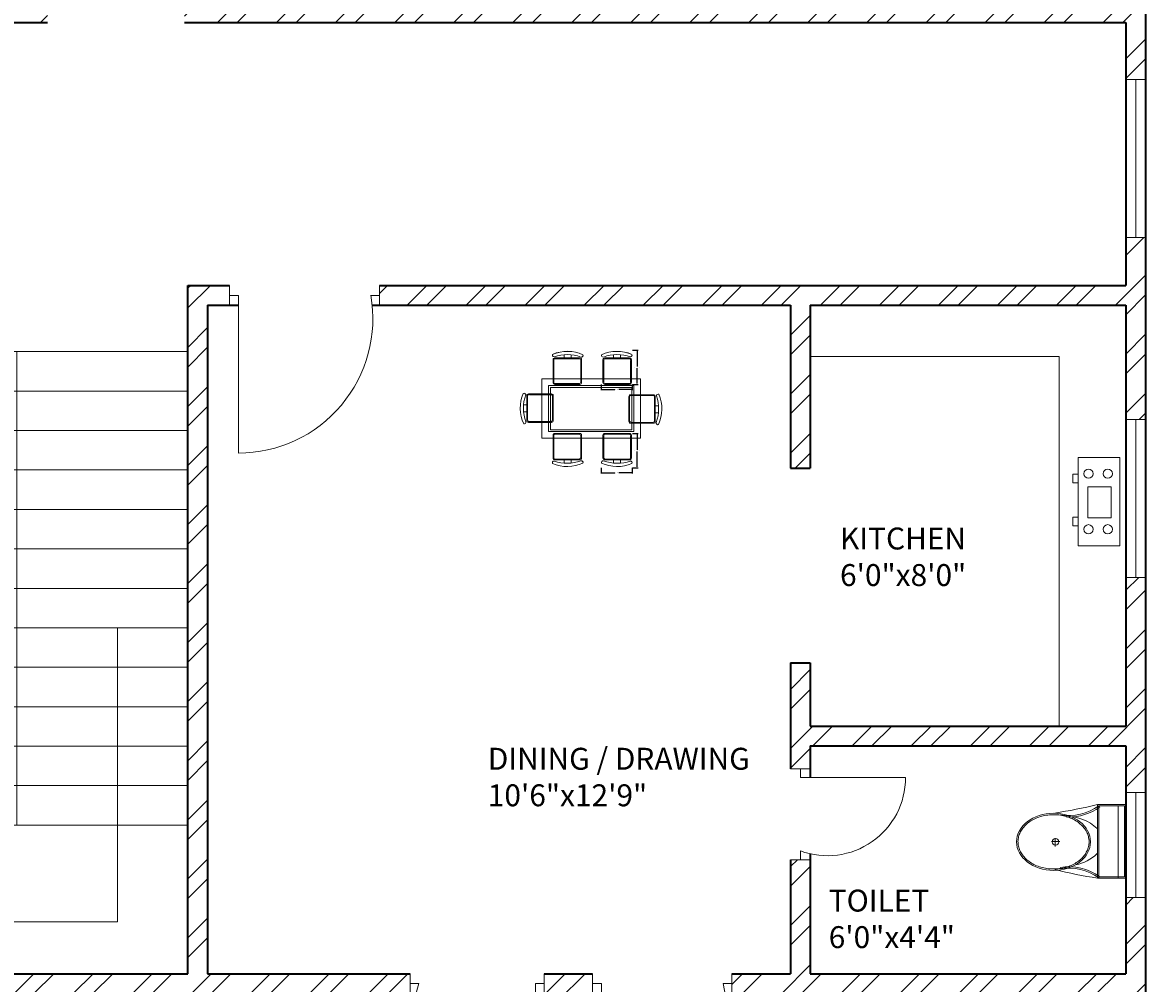
# Model space of a CAD drawing. Units: inches. Extents: x 1944 to 3454, y 1352 to 3055.
# Tile 4 of 17: x 2314 to 2570, y 1681 to 1900. Entities that reach past the tile are written whole.
import ezdxf

# ---------------------------------------------------------------- set-up
doc = ezdxf.new("R2010")
doc.units = ezdxf.units.IN
for name, color, linetype, lineweight in [('A-ANNO-DIMS', 2, 'Continuous', 18), ('A-AREA-IDEN', 7, 'Continuous', 18), ('A-DOOR', 3, 'Continuous', 20), ('A-EQPM', 9, 'Continuous', 18), ('A-FLOR-CASE', 8, 'Continuous', 20), ('A-FLOR-FIXT', 9, 'Continuous', 18), ('A-FLOR-STRS', 7, 'Continuous', 20), ('A-FURN', 8, 'Continuous', 13), ('A-GLAZ', 4, 'Continuous', 18), ('A-WALL', 7, 'Continuous', 35), ('A-WALL-PATT', 252, 'Continuous', 13)]:
    doc.layers.add(name, color=color, linetype=linetype, lineweight=lineweight)
doc.styles.get("Standard").update_dxf_attribs({"font": 'arial.ttf'})
doc.dimstyles.get("Standard").update_dxf_attribs({"dimtxt": 0.18, "dimasz": 0.18, "dimexe": 0.18, "dimexo": 0.0625, "dimgap": 0.09, "dimtad": 0, "dimtih": 1, "dimtoh": 1, "dimdec": 4, "dimzin": 0, "dimdsep": 46, "dimtxsty": 'Standard', "dimcen": 0.09, "dimadec": 0, "dimazin": 0, "dimtfac": 1, "dimtdec": 4, "dimtofl": 0, "dimtmove": 0, "dimatfit": 3, "dimfxl": 1, "dimtolj": 1, "dimtzin": 0, "dimarcsym": 0})

# ---------------------------------------------------------------- blocks, each defined once
blk = doc.blocks.new('A$C31115884')
for p, q in [((283.1, 497.7), (223.4, 497.7)), ((257.5, 466.4), (257.5, 523.2)), ((0, 200), (0, 0)), ((520, 200), (0, 200)), ((10, 190), (10, 10)), ((510, 190), (10, 190)), ((510, 10), (510, 190)), ((520, 0), (520, 200)), ((510, 54.5), (0, 54.5)), ((10, 10), (510, 10)), ((0, 0), (520, 0))]:
    blk.add_line(p, q)
blk.add_circle((255.6, 496.4), 23.6)
for centre, radius, start, end in [((2777.7, -204.6), 2807, 165.4549, 171.71327), ((3237, 905), 2807, 188.28673, 194.5451), ((-294.5, 403.3), 364.7, 324.20913, 9.34987), ((-294.5, 403.3), 374.7, 324.20913, 9.34987), ((139.5, 406.2), 293.5, 315.84364, 2.65635), ((805.8, 403.3), 374.7, 179.20365, 215.79087), ((805.8, 403.3), 364.7, 170.65013, 215.79087), ((383.6, 406.2), 293.5, 190.27735, 224.15636)]:
    blk.add_arc(centre, radius, start, end)
blk.add_ellipse((256.2, 509.9), major_axis=(0, -260.7), ratio=0.772727)
blk.add_open_spline([(256.2, 259.2), (263.1, 259.2), (270, 259.7), (287.8, 262.3), (298.7, 265.1), (319.9, 273.1), (330.2, 278.4), (350.1, 291.1), (359.7, 298.7), (377.7, 315.9), (386.2, 325.5), (401.7, 346.6), (408.8, 358.1), (421.3, 382.5), (426.8, 395.5), (435.9, 422.4), (439.5, 436.4), (444.8, 465.1), (446.5, 479.7), (447.9, 509.2), (447.6, 524), (445, 553.3), (442.7, 567.8), (436.3, 596), (432.1, 609.7), (421.9, 636), (416, 648.6), (402.5, 672.1), (395, 683), (378.6, 703), (369.8, 712.1), (351.1, 728), (341.3, 734.8), (320.9, 746.2), (310.4, 750.7), (288.9, 757.3), (278, 759.4), (256, 761), (245, 760.6), (223.1, 757.2), (212.3, 754.3), (191.1, 746.1), (180.8, 740.7), (160.9, 727.8), (151.4, 720.1), (133.5, 702.7), (125.1, 693), (109.6, 671.7), (102.6, 660.2), (90.2, 635.7), (84.9, 622.7), (76, 595.6), (72.4, 581.6), (67.2, 552.9), (65.6, 538.2), (64.4, 508.8), (64.8, 494), (67.5, 464.7), (69.9, 450.2), (76.6, 422), (80.8, 408.3), (91.1, 382.2), (97.2, 369.7), (110.8, 346.3), (118.4, 335.4), (134.8, 315.6), (143.7, 306.7), (162.4, 290.9), (172.3, 284.2), (192.8, 273), (203.3, 268.6), (224.8, 262.2), (235.8, 260.2), (249.9, 259.3), (253, 259.2), (256.2, 259.2)], degree=3, knots=[0, 0, 0, 0, 0.110105, 0.110105, 0.285049, 0.285049, 0.459994, 0.459994, 0.634938, 0.634938, 0.809882, 0.809882, 0.984827, 0.984827, 1.159771, 1.159771, 1.334715, 1.334715, 1.50966, 1.50966, 1.684604, 1.684604, 1.859549, 1.859549, 2.034493, 2.034493, 2.209437, 2.209437, 2.384382, 2.384382, 2.559326, 2.559326, 2.73427, 2.73427, 2.909215, 2.909215, 3.084159, 3.084159, 3.259103, 3.259103, 3.434048, 3.434048, 3.608992, 3.608992, 3.783936, 3.783936, 3.958881, 3.958881, 4.133825, 4.133825, 4.30877, 4.30877, 4.483714, 4.483714, 4.658658, 4.658658, 4.833603, 4.833603, 5.008547, 5.008547, 5.183491, 5.183491, 5.358436, 5.358436, 5.53338, 5.53338, 5.708324, 5.708324, 5.883269, 5.883269, 6.058213, 6.058213, 6.233158, 6.233158, 6.283185, 6.283185, 6.283185, 6.283185])
blk = doc.blocks.new('COOKTOP-4B-01')
for points in [[(0, 20.18), (9.48, 20.18), (9.48, 0), (0, 0)], [(9.48, 15.59), (10.71, 15.59), (10.71, 13.59), (9.48, 13.59)], [(2, 13.79), (7.26, 13.79), (7.26, 6.73), (2, 6.73)], [(9.48, 5.81), (10.71, 5.81), (10.71, 3.8), (9.48, 3.8)]]:
    blk.add_lwpolyline(points, close=True)
for centre in [(2.74, 16.38), (7.14, 16.38), (2.74, 3.71), (7.14, 3.71)]:
    blk.add_circle(centre, 1.05)
blk = doc.blocks.new('DOOR-SWING-24IN-07')
for p, q in [((4.5, 20.75), (0, 20.75)), ((0, 20.75), (2.25, 20.75)), ((2.25, 20.75), (2.25, 18.75)), ((2.25, 18.75), (26.25, 18.75)), ((4.5, 0), (0, 0)), ((0, 0), (2.25, 0)), ((2.25, 0), (2.25, 2))]:
    blk.add_line(p, q)
blk.add_arc((8.4, 18.75), 17.84, 249.8228, 0)
blk = doc.blocks.new('DOOR-SWING-36IN-05')
for p, q in [((0, 33.75), (0, 38.25)), ((0, 38.25), (0, 36)), ((0, 36), (0, 36)), ((0, 36), (2, 36)), ((2, 36), (2, 0)), ((31.76, 36), (29.76, 36)), ((31.76, 33.75), (31.76, 38.25)), ((31.76, 38.25), (31.76, 36))]:
    blk.add_line(p, q)
blk.add_arc((2, 28.7), 28.7, 270, 14.7288)
blk = doc.blocks.new('DOOR-SWING-36IN-06')
for p, q in [((0, 33.75), (0, 38.25)), ((0, 38.25), (0, 36)), ((0, 36), (2, 36)), ((30.6, 36), (28.6, 36)), ((28.6, 36), (28.6, 0)), ((30.6, 33.75), (30.6, 38.25)), ((30.6, 38.25), (30.6, 36))]:
    blk.add_line(p, q)
blk.add_arc((28.6, 27.83), 27.83, 162.9212, 270)
blk = doc.blocks.new('DOOR-SWING-36IN-12')
for p, q in [((0, 33.75), (0, 38.25)), ((0, 38.25), (0, 36)), ((0, 36), (2, 36)), ((2, 36), (2, 0)), ((34.2, 36), (32.2, 36)), ((34.2, 33.75), (34.2, 38.25)), ((34.2, 38.25), (34.2, 36))]:
    blk.add_line(p, q)
blk.add_arc((2, 30.67), 30.67, 270, 10.0117)
blk = doc.blocks.new('WINDOW-PLAN-36.00IN-01')
for p, q in [((0, 36), (4.5, 36)), ((4.5, 36), (2.25, 36)), ((2.25, 36), (2.25, 0)), ((2.25, 0), (0, 0)), ((0, 0), (4.5, 0))]:
    blk.add_line(p, q)
blk = doc.blocks.new('WINDOW-PLAN-24.00IN-02')
for p, q in [((0, 24), (4.5, 24)), ((4.5, 24), (2.25, 24)), ((2.25, 24), (2.25, 0)), ((4.5, 0), (0, 0)), ((2.25, 0), (4.5, 0))]:
    blk.add_line(p, q)
blk = doc.blocks.new('STAIR-TWO-FLIGHT-01')
for p, q in [((18.12, 152.99), (18.12, 0)), ((0, 130.08), (78, 130.08)), ((78, 130.08), (39, 130.08)), ((39, 130.08), (39, 22.08)), ((0, 121.08), (78, 121.08)), ((0, 112.08), (78, 112.08)), ((0, 103.08), (78, 103.08)), ((0, 94.08), (78, 94.08)), ((0, 85.08), (78, 85.08)), ((0, 76.08), (78, 76.08)), ((0, 67.08), (78, 67.08)), ((61.93, 0), (61.93, 67.08)), ((0, 58.08), (78, 58.08)), ((0, 49.08), (78, 49.08)), ((0, 40.08), (78, 40.08)), ((0, 31.08), (78, 31.08)), ((0, 22.08), (78, 22.08)), ((18.12, 0), (61.93, 0))]:
    blk.add_line(p, q)
blk = doc.blocks.new('TABLE-DINING-01')
for points in [[(0, 13.51), (22.52, 13.51), (22.52, 0), (0, 0)], [(0, 13.51), (22.52, 13.51), (22.52, 0), (0, 0)], [(1.5, 12.01), (21.02, 12.01), (21.02, 1.5), (1.5, 1.5)], [(1.5, 12.01), (21.02, 12.01), (21.02, 1.5), (1.5, 1.5)], [(1.95, 11.56), (20.57, 11.56), (20.57, 1.95), (1.95, 1.95)], [(1.95, 11.56), (20.57, 11.56), (20.57, 1.95), (1.95, 1.95)]]:
    blk.add_lwpolyline(points, close=True)
blk = doc.blocks.new('CHAIR-DINING-02')
for points in [[(0.48, 6.23, -0.578392), (0.02, 6.74, -0.214524), (6.94, 6.84, -0.552014), (6.62, 6.28, 0.175809), (0.48, 6.23)], [(6.44, 6.03, -0.414214), (6.84, 5.63), (6.84, 0.4, -0.414214), (6.44, 0), (0.74, 0, -0.414214), (0.34, 0.4), (0.34, 5.63, -0.414214), (0.74, 6.03), (6.44, 6.03)], [(2.74, 6.03), (2.74, 6.75, 0.064759)]]:
    blk.add_lwpolyline(points, format="xyb")
blk.add_lwpolyline([(6.44, 5.85), (0.92, 5.85, 0.414214), (0.52, 5.45), (0.52, 0.58, 0.414214), (0.92, 0.18), (6.44, 0.18, 0.512069), (6.66, 0.58), (6.66, 5.45, 0.512069)], format="xyb", close=True)
blk.add_lwpolyline([(4.34, 6.77), (4.34, 6.03)])
blk = doc.blocks.new('CHAIR-DINING-04')
for points in [[(6.24, 1.5), (0.55, 1.5, -0.414214), (0.15, 1.9), (0.15, 7.13, -0.414214), (0.55, 7.53), (6.24, 7.53, -0.414214), (6.64, 7.13), (6.64, 1.9, -0.414214), (6.24, 1.5)], [(6.5, 1.3, -0.578392), (6.97, 0.79, -0.214524), (0.04, 0.7, -0.552014), (0.37, 1.25, 0.175809), (6.5, 1.3)], [(4.24, 1.5), (4.24, 0.78, 0.064759)]]:
    blk.add_lwpolyline(points, format="xyb")
blk.add_lwpolyline([(0.55, 1.68), (6.06, 1.68, 0.414214), (6.46, 2.08), (6.46, 6.95, 0.414214), (6.06, 7.35), (0.55, 7.35, 0.512069), (0.33, 6.95), (0.33, 2.08, 0.512069)], format="xyb", close=True)
blk.add_lwpolyline([(2.65, 0.77), (2.65, 1.5)])
blk = doc.blocks.new('CHAIR-DINING-06')
for points in [[(0.37, 6.28, -0.175809), (6.5, 6.23, 0.578392), (6.97, 6.74, 0.214524), (0.04, 6.84, 0.552014), (0.37, 6.28, -0.065079)], [(6.24, 6.03), (0.55, 6.03, 0.414214), (0.15, 5.63), (0.15, 0.4, 0.414214), (0.55, 0), (6.24, 0, 0.414214), (6.64, 0.4), (6.64, 5.63, 0.414214), (6.24, 6.03)], [(4.24, 6.03), (4.24, 6.75, -0.064759)]]:
    blk.add_lwpolyline(points, format="xyb")
blk.add_lwpolyline([(0.55, 5.85), (6.06, 5.85, -0.414214), (6.46, 5.46), (6.46, 0.58, -0.414214), (6.06, 0.18), (0.55, 0.18, -0.512069), (0.33, 0.58), (0.33, 5.46, -0.512069)], format="xyb", close=True)
blk.add_lwpolyline([(2.65, 6.77), (2.65, 6.03)])
blk = doc.blocks.new('CHAIR-DINING-07')
for points in [[(1.3, 0.48, -0.578392), (0.79, 0.02, -0.214524), (0.7, 6.94, -0.552014), (1.25, 6.62, 0.175809), (1.3, 0.48)], [(1.5, 6.44, -0.414214), (1.9, 6.84), (7.13, 6.84, -0.414214), (7.53, 6.44), (7.53, 0.74, -0.414214), (7.13, 0.34), (1.9, 0.34, -0.414214), (1.5, 0.74), (1.5, 6.44)], [(1.5, 2.74), (0.78, 2.74, 0.064759)]]:
    blk.add_lwpolyline(points, format="xyb")
blk.add_lwpolyline([(1.68, 6.44), (1.68, 0.92, 0.414214), (2.08, 0.52), (6.95, 0.52, 0.414214), (7.35, 0.92), (7.35, 6.44, 0.512069), (6.95, 6.66), (2.08, 6.66, 0.512069)], format="xyb", close=True)
blk.add_lwpolyline([(0.77, 4.34), (1.5, 4.34)])
blk = doc.blocks.new('CHAIR-DINING-08')
for points in [[(1.3, 0.48, -0.578392), (0.79, 0.02, -0.214524), (0.7, 6.94, -0.552014), (1.25, 6.62, 0.175809), (1.3, 0.48)], [(1.5, 6.44, -0.414214), (1.9, 6.84), (7.13, 6.84, -0.414214), (7.53, 6.44), (7.53, 0.74, -0.414214), (7.13, 0.35), (1.9, 0.35, -0.414214), (1.5, 0.74), (1.5, 6.44)], [(1.5, 2.74), (0.78, 2.74, 0.064759)]]:
    blk.add_lwpolyline(points, format="xyb")
blk.add_lwpolyline([(1.68, 6.44), (1.68, 0.92, 0.414214), (2.08, 0.52), (6.95, 0.52, 0.414214), (7.35, 0.92), (7.35, 6.44, 0.512069), (6.95, 6.66), (2.08, 6.66, 0.512069)], format="xyb", close=True)
blk.add_lwpolyline([(0.77, 4.34), (1.5, 4.34)])
blk = doc.blocks.new('CHAIR-DINING-10')
for points in [[(6.44, 1.5, 0.414214), (6.84, 1.9), (6.84, 7.13, 0.414214), (6.44, 7.53), (0.74, 7.53, 0.414214), (0.34, 7.13), (0.34, 1.9, 0.414214), (0.74, 1.5), (6.44, 1.5)], [(6.62, 1.25, -0.175809), (0.48, 1.3, 0.578392), (0.02, 0.79, 0.214524), (6.94, 0.7, 0.552014), (6.62, 1.25, -0.065079)], [(2.74, 1.5), (2.74, 0.78, -0.064759)]]:
    blk.add_lwpolyline(points, format="xyb")
blk.add_lwpolyline([(6.44, 1.68), (0.92, 1.68, -0.414214), (0.52, 2.08), (0.52, 6.95, -0.414214), (0.92, 7.35), (6.44, 7.35, -0.512069), (6.66, 6.95), (6.66, 2.08, -0.512069)], format="xyb", close=True)
blk.add_lwpolyline([(4.34, 0.77), (4.34, 1.5)])
blk = doc.blocks.new('CHAIR-DINING-11')
for points in [[(6.44, 1.5, 0.414214), (6.84, 1.9), (6.84, 7.13, 0.414214), (6.44, 7.53), (0.74, 7.53, 0.414214), (0.34, 7.13), (0.34, 1.9, 0.414214), (0.74, 1.5), (6.44, 1.5)], [(6.62, 1.25, -0.175809), (0.48, 1.3, 0.578392), (0.02, 0.79, 0.214524), (6.94, 0.7, 0.552014), (6.62, 1.25, -0.065079)], [(2.74, 1.5), (2.74, 0.78, -0.064759)]]:
    blk.add_lwpolyline(points, format="xyb")
blk.add_lwpolyline([(6.44, 1.68), (0.92, 1.68, -0.414214), (0.52, 2.08), (0.52, 6.95, -0.414214), (0.92, 7.35), (6.44, 7.35, -0.512069), (6.66, 6.95), (6.66, 2.08, -0.512069)], format="xyb", close=True)
blk.add_lwpolyline([(4.34, 0.77), (4.34, 1.5)])
blk = doc.blocks.new('*D142')
at = {"layer": 'A-ANNO-DIMS', "color": 0, "lineweight": -2, "transparency": 16777216}
for p, q in [((2452.74, 1825.34), (2454.03, 1825.34)), ((2453.85, 1825.16), (2453.85, 1821.62)), ((2453.85, 1817.72), (2453.85, 1821.25)), ((2452.74, 1817.54), (2454.03, 1817.54))]:
    blk.add_line(p, q, dxfattribs=at)
at = {"layer": 'A-ANNO-DIMS', "color": 0, "transparency": 16777216}
for points in [[(2453.82, 1825.16), (2453.88, 1825.16), (2453.85, 1825.34)], [(2453.82, 1817.72), (2453.88, 1817.72), (2453.85, 1817.54)]]:
    blk.add_solid(points, dxfattribs=at)
at = {"layer": 'Defpoints', "color": 0, "transparency": 16777216}
for p in [(2452.68, 1825.34), (2453.85, 1825.34), (2452.68, 1817.54)]:
    blk.add_point(p, dxfattribs=at)
at = {"layer": 'A-ANNO-DIMS', "color": 0, "transparency": 16777216, "insert": (2453.85, 1821.44), "char_height": 0.18, "attachment_point": 5}
blk.add_mtext('\\A1;CHAIR 8 TYP.', dxfattribs=at)
blk = doc.blocks.new('*D143')
at = {"layer": 'A-ANNO-DIMS', "color": 0, "lineweight": -2, "transparency": 16777216}
for p, q in [((2445.65, 1817.48), (2445.65, 1816.19)), ((2452.68, 1817.48), (2452.68, 1816.19)), ((2445.83, 1816.37), (2448.71, 1816.37)), ((2452.5, 1816.37), (2449.62, 1816.37))]:
    blk.add_line(p, q, dxfattribs=at)
at = {"layer": 'A-ANNO-DIMS', "color": 0, "transparency": 16777216}
for points in [[(2445.83, 1816.4), (2445.83, 1816.34), (2445.65, 1816.37)], [(2452.5, 1816.4), (2452.5, 1816.34), (2452.68, 1816.37)]]:
    blk.add_solid(points, dxfattribs=at)
at = {"layer": 'Defpoints', "color": 0, "transparency": 16777216}
for p in [(2445.65, 1817.54), (2452.68, 1817.54), (2452.68, 1816.37)]:
    blk.add_point(p, dxfattribs=at)
at = {"layer": 'A-ANNO-DIMS', "color": 0, "transparency": 16777216, "insert": (2449.16, 1816.37), "char_height": 0.18, "attachment_point": 5}
blk.add_mtext('\\A1;7 TYP.', dxfattribs=at)
blk = doc.blocks.new('*D160')
at = {"layer": 'A-ANNO-DIMS', "color": 0, "lineweight": -2, "transparency": 16777216}
for p, q in [((2452.74, 1806.33), (2454.03, 1806.33)), ((2453.85, 1806.15), (2453.85, 1802.61)), ((2453.85, 1798.71), (2453.85, 1802.25)), ((2452.74, 1798.53), (2454.03, 1798.53))]:
    blk.add_line(p, q, dxfattribs=at)
at = {"layer": 'A-ANNO-DIMS', "color": 0, "transparency": 16777216}
for points in [[(2453.82, 1806.15), (2453.88, 1806.15), (2453.85, 1806.33)], [(2453.82, 1798.71), (2453.88, 1798.71), (2453.85, 1798.53)]]:
    blk.add_solid(points, dxfattribs=at)
at = {"layer": 'Defpoints', "color": 0, "transparency": 16777216}
for p in [(2452.68, 1806.33), (2453.85, 1806.33), (2452.68, 1798.53)]:
    blk.add_point(p, dxfattribs=at)
at = {"layer": 'A-ANNO-DIMS', "color": 0, "transparency": 16777216, "insert": (2453.85, 1802.43), "char_height": 0.18, "attachment_point": 5}
blk.add_mtext('\\A1;CHAIR 8 TYP.', dxfattribs=at)
blk = doc.blocks.new('*D161')
at = {"layer": 'A-ANNO-DIMS', "color": 0, "lineweight": -2, "transparency": 16777216}
for p, q in [((2445.65, 1798.47), (2445.65, 1797.18)), ((2445.83, 1797.36), (2448.71, 1797.36)), ((2452.5, 1797.36), (2449.62, 1797.36)), ((2452.68, 1798.47), (2452.68, 1797.18))]:
    blk.add_line(p, q, dxfattribs=at)
at = {"layer": 'A-ANNO-DIMS', "color": 0, "transparency": 16777216}
for points in [[(2445.83, 1797.39), (2445.83, 1797.33), (2445.65, 1797.36)], [(2452.5, 1797.39), (2452.5, 1797.33), (2452.68, 1797.36)]]:
    blk.add_solid(points, dxfattribs=at)
at = {"layer": 'Defpoints', "color": 0, "transparency": 16777216}
for p in [(2445.65, 1798.53), (2452.68, 1798.53), (2452.68, 1797.36)]:
    blk.add_point(p, dxfattribs=at)
at = {"layer": 'A-ANNO-DIMS', "color": 0, "transparency": 16777216, "insert": (2449.16, 1797.36), "char_height": 0.18, "attachment_point": 5}
blk.add_mtext('\\A1;7 TYP.', dxfattribs=at)

msp = doc.modelspace()

# ---------------------------------------------------------------- hatches: boundary and pattern name
at = {"layer": 'A-WALL-PATT'}
h = msp.add_hatch(dxfattribs=at)
h.set_pattern_fill('ANSI32', color=256)
h.paths.add_polyline_path([(2061.822, 2177.596), (2158.181, 2177.596), (2158.181, 2179.846), (2158.181, 2182.096), (2057.322, 2182.096), (2057.322, 2123.452), (2061.822, 2123.452)])
h.paths.add_polyline_path([(2258.993, 2179.846), (2258.993, 2182.096), (2218.838, 2182.096), (2218.838, 2177.596), (2258.993, 2177.596)])
h.paths.add_polyline_path([(2315.822, 2177.596), (2322.722, 2177.596), (2322.722, 2182.096), (2303.186, 2182.096), (2303.186, 2177.596), (2311.322, 2177.596), (2311.322, 2033.596), (2231.355, 2033.596), (2231.355, 2029.096), (2311.322, 2029.096), (2311.322, 1904.596), (2307.941, 1904.596), (2307.941, 1900.096), (2319.277, 1900.096), (2319.277, 1902.346), (2319.277, 1904.596), (2315.822, 1904.596), (2315.822, 2029.096), (2394.855, 2029.096), (2394.855, 2033.596), (2315.822, 2033.596)])
h.paths.add_polyline_path([(2407.334, 2182.096), (2366.1, 2182.096), (2366.1, 2177.596), (2407.334, 2177.596), (2407.334, 2179.846)])
h.paths.add_polyline_path([(2440.322, 2177.596), (2443.866, 2177.596), (2443.866, 2182.096), (2431.827, 2182.096), (2431.827, 2179.846), (2431.827, 2177.596), (2435.822, 2177.596), (2435.822, 2033.596), (2430.464, 2033.596), (2430.464, 2029.096), (2445.372, 2029.096), (2445.372, 2031.346), (2445.372, 2033.596), (2440.322, 2033.596)])
h.paths.add_polyline_path([(2569.822, 2182.096), (2466.481, 2182.096), (2466.481, 2177.596), (2565.322, 2177.596), (2565.322, 2123.452), (2569.822, 2123.452)])
h.paths.add_polyline_path([(2569.822, 2063.452), (2567.572, 2063.452), (2565.322, 2063.452), (2565.322, 2033.596), (2478.08, 2033.596), (2476.822, 2033.596), (2476.822, 2028.698), (2476.822, 2020.069), (2481.322, 2020.069), (2481.322, 2029.096), (2565.322, 2029.096), (2565.322, 2014.5), (2569.822, 2014.5)])
h.paths.add_polyline_path([(2569.822, 1978.5), (2565.322, 1978.5), (2565.322, 1957.096), (2481.322, 1957.096), (2481.322, 1990.369), (2476.822, 1990.369), (2476.822, 1957.096), (2476.822, 1952.596), (2476.822, 1947.471), (2481.322, 1947.471), (2481.322, 1952.596), (2565.322, 1952.596), (2565.322, 1943.2), (2569.822, 1943.2)])
h.paths.add_polyline_path([(2569.822, 1919.2), (2565.322, 1919.2), (2565.322, 1904.596), (2481.322, 1904.596), (2481.322, 1928.596), (2476.822, 1928.596), (2476.822, 1904.596), (2350.518, 1904.596), (2350.518, 1900.096), (2476.822, 1900.096), (2565.322, 1900.096), (2565.322, 1895.596), (2565.322, 1887.047), (2569.822, 1887.047)])
h.paths.add_polyline_path([(2280.492, 1904.596), (2150.322, 1904.596), (2150.322, 1926.68), (2148.072, 1926.68), (2145.822, 1926.68), (2145.822, 1904.596), (2061.822, 1904.596), (2061.822, 1914.977), (2059.572, 1914.977), (2057.322, 1914.977), (2057.322, 1887.362), (2061.822, 1887.362), (2061.822, 1900.096), (2150.322, 1900.096), (2280.492, 1900.096), (2280.492, 1902.346)])
h.paths.add_polyline_path([(2150.322, 1957.096), (2150.322, 1986.22), (2145.822, 1986.22), (2145.822, 1957.096), (2061.822, 1957.096), (2061.822, 1975.678), (2057.322, 1975.678), (2057.322, 1938.977), (2061.822, 1938.977), (2061.822, 1952.596), (2145.822, 1952.596), (2145.822, 1947.985), (2150.322, 1947.985), (2150.322, 1952.596)])
h.paths.add_polyline_path([(2061.822, 2063.452), (2057.322, 2063.452), (2057.322, 2011.678), (2061.822, 2011.678), (2061.822, 2029.096), (2145.288, 2029.096), (2145.822, 2029.096), (2145.822, 2019.118), (2150.322, 2019.118), (2150.322, 2029.096), (2150.322, 2033.596), (2147.022, 2033.596), (2061.822, 2033.596)])
h.paths.add_polyline_path([(2061.822, 1835.596), (2133.822, 1835.596), (2133.822, 1794.415), (2138.322, 1794.415), (2138.322, 1835.596), (2231.726, 1835.596), (2231.726, 1840.096), (2061.822, 1840.096), (2061.822, 1851.362), (2057.322, 1851.362), (2057.322, 1810.528), (2061.822, 1810.528)])
h.paths.add_polyline_path([(2061.822, 1774.528), (2059.572, 1774.528), (2057.322, 1774.528), (2057.322, 1723.746), (2061.822, 1723.746), (2061.822, 1735.096), (2133.822, 1735.096), (2133.822, 1731.415), (2138.322, 1731.415), (2138.322, 1759.737), (2133.822, 1759.737), (2133.822, 1739.596), (2061.822, 1739.596)])
h.paths.add_polyline_path([(2061.822, 1678.596), (2147.597, 1678.596), (2147.597, 1680.846), (2147.597, 1683.096), (2138.322, 1683.096), (2138.322, 1710.66), (2136.072, 1710.66), (2133.822, 1710.66), (2133.822, 1683.096), (2061.822, 1683.096), (2061.822, 1699.746), (2057.322, 1699.746), (2057.322, 1645.751), (2061.822, 1645.751)])
h.paths.add_polyline_path([(2061.822, 1585.751), (2057.322, 1585.751), (2057.322, 1530.096), (2158.703, 1530.096), (2158.703, 1534.596), (2061.822, 1534.596)])
h.paths.add_polyline_path([(2191.322, 1678.596), (2195.889, 1678.596), (2195.889, 1683.096), (2181.763, 1683.096), (2181.763, 1680.846), (2181.763, 1678.596), (2186.822, 1678.596), (2186.822, 1534.596), (2181.354, 1534.596), (2181.354, 1530.096), (2196.54, 1530.096), (2196.54, 1532.346), (2196.54, 1534.596), (2191.322, 1534.596)])
h.paths.add_polyline_path([(2315.822, 1678.596), (2402.014, 1678.596), (2402.014, 1683.096), (2355.822, 1683.096), (2355.822, 1835.596), (2360.838, 1835.596), (2360.838, 1840.096), (2351.322, 1840.096), (2351.322, 1683.096), (2273.322, 1683.096), (2273.322, 1840.096), (2263.134, 1840.096), (2263.134, 1837.846), (2263.134, 1835.596), (2268.822, 1835.596), (2268.822, 1683.096), (2227.793, 1683.096), (2227.793, 1678.596), (2311.322, 1678.596), (2311.322, 1534.596), (2302.384, 1534.596), (2302.384, 1530.096), (2324.521, 1530.096), (2324.521, 1532.346), (2324.521, 1534.596), (2315.822, 1534.596)])
h.paths.add_polyline_path([(2440.322, 1678.596), (2443.656, 1678.596), (2443.656, 1683.096), (2432.614, 1683.096), (2432.614, 1680.846), (2432.614, 1678.596), (2435.822, 1678.596), (2435.822, 1534.596), (2440.322, 1534.596)])
h.paths.add_polyline_path([(2409.913, 1534.596), (2369.033, 1534.596), (2369.033, 1530.096), (2409.913, 1530.096)])
h.paths.add_polyline_path([(2259.529, 1532.346), (2259.529, 1534.596), (2218.889, 1534.596), (2218.889, 1532.346), (2218.889, 1530.096), (2259.529, 1530.096)])
h.paths.add_polyline_path([(2569.822, 1584.389), (2567.572, 1584.389), (2565.322, 1584.389), (2565.322, 1534.596), (2465.892, 1534.596), (2465.892, 1530.096), (2569.822, 1530.096)])
h.paths.add_polyline_path([(2505.567, 1530.096), (2501.067, 1530.096), (2501.067, 1494.096), (2381.067, 1494.096), (2381.067, 1530.096), (2376.567, 1530.096), (2376.567, 1489.596), (2381.067, 1489.596), (2505.567, 1489.596), (2505.567, 1494.096)])
h.paths.add_polyline_path([(2127.673, 1530.096), (2123.173, 1530.096), (2123.173, 1489.596), (2127.673, 1489.596), (2252.173, 1489.596), (2252.173, 1494.096), (2252.173, 1530.096), (2247.673, 1530.096), (2247.673, 1494.096), (2127.673, 1494.096)])
h.paths.add_polyline_path([(2251.167, 2222.596), (2126.667, 2222.596), (2122.167, 2222.596), (2122.167, 2182.096), (2126.667, 2182.096), (2126.667, 2218.096), (2210.667, 2218.096), (2234.667, 2218.096), (2246.667, 2218.096), (2246.667, 2182.096), (2251.167, 2182.096), (2251.167, 2218.096)])
h.paths.add_polyline_path([(2501.916, 2222.596), (2497.416, 2222.596), (2372.916, 2222.596), (2372.916, 2218.096), (2372.916, 2182.096), (2377.416, 2182.096), (2377.416, 2218.096), (2497.416, 2218.096), (2497.416, 2182.096), (2501.916, 2182.096)])
h.paths.add_polyline_path([(2569.822, 1700.442), (2565.322, 1700.442), (2565.322, 1683.096), (2493.322, 1683.096), (2493.322, 1709.096), (2488.822, 1709.096), (2488.822, 1683.096), (2475.416, 1683.096), (2475.416, 1680.846), (2475.416, 1678.596), (2488.822, 1678.596), (2565.322, 1678.596), (2565.322, 1644.389), (2569.822, 1644.389)])
h.paths.add_polyline_path([(2569.822, 1773.506), (2565.322, 1773.506), (2565.322, 1739.596), (2493.322, 1739.596), (2493.322, 1754.002), (2488.822, 1754.002), (2488.822, 1729.846), (2491.072, 1729.846), (2493.322, 1729.846), (2493.322, 1735.096), (2565.322, 1735.096), (2565.322, 1724.442), (2569.822, 1724.442)])
h.paths.add_polyline_path([(2569.822, 1851.047), (2567.572, 1851.047), (2565.322, 1851.047), (2565.322, 1840.096), (2395.039, 1840.096), (2395.039, 1837.846), (2395.039, 1835.596), (2488.822, 1835.596), (2488.822, 1798.423), (2493.322, 1798.423), (2493.322, 1835.596), (2565.322, 1835.596), (2565.322, 1809.506), (2569.822, 1809.506)])
h.paths.add_polyline_path([(2347.275, 1955.576), (2414.024, 1955.576), (2414.024, 1974.234), (2347.275, 1974.234)], flags=9)
h.paths.add_polyline_path([(2509.756, 1990.497), (2542.915, 1990.497), (2542.915, 2009.154), (2509.756, 2009.154)], flags=9)

# ---------------------------------------------------------------- linework, layer by layer
at = {"layer": 'A-FLOR-CASE'}
for p, q in [((2493.322, 1823.863), (2550.107, 1823.863)), ((2550.107, 1823.863), (2550.107, 1739.596))]:
    msp.add_line(p, q, dxfattribs=at)
at = {"layer": 'A-FURN'}
for points in [[(2434.861, 1823.817, -0.1758092), (2440.995, 1823.771, 0.5783921), (2441.46, 1824.282, 0.2145244), (2434.536, 1824.375, 0.552014), (2434.861, 1823.817, -0.065079)], [(2446.159, 1823.771, -0.5783921), (2445.694, 1824.282, -0.2145244), (2452.618, 1824.375, -0.552014), (2452.293, 1823.817, 0.1758092), (2446.159, 1823.771)], [(2440.735, 1823.571), (2435.04, 1823.571, 0.4142136), (2434.642, 1823.173), (2434.642, 1817.937, 0.4142136), (2435.04, 1817.538), (2440.735, 1817.538, 0.4142136), (2441.133, 1817.937), (2441.133, 1823.173, 0.4142136), (2440.735, 1823.571)], [(2438.735, 1823.571), (2438.735, 1824.291, -0.0647586)], [(2452.114, 1823.571, -0.4142136), (2452.512, 1823.173), (2452.512, 1817.937, -0.4142136), (2452.114, 1817.538), (2446.419, 1817.538, -0.4142136), (2446.021, 1817.937), (2446.021, 1823.173, -0.4142136), (2446.419, 1823.571), (2452.114, 1823.571)], [(2448.419, 1823.571), (2448.419, 1824.291, 0.0647586)], [(2457.967, 1814.765, 0.4142136), (2457.569, 1815.163), (2452.333, 1815.163, 0.4142136), (2451.935, 1814.765), (2451.935, 1809.07, 0.4142136), (2452.333, 1808.672), (2457.569, 1808.672, 0.4142136), (2457.967, 1809.07), (2457.967, 1814.765)], [(2457.967, 1814.765, 0.4142136), (2457.569, 1815.163), (2452.333, 1815.163, 0.4142136), (2451.935, 1814.765), (2451.935, 1809.07, 0.4142136), (2452.333, 1808.672), (2457.569, 1808.672, 0.4142136), (2457.967, 1809.07), (2457.967, 1814.765)], [(2458.214, 1814.944, -0.1758092), (2458.167, 1808.81, 0.5783921), (2458.678, 1808.346, 0.2145244), (2458.771, 1815.269, 0.552014), (2458.214, 1814.944, -0.065079)], [(2458.214, 1814.944, -0.1758092), (2458.167, 1808.81, 0.5783921), (2458.678, 1808.345, 0.2145244), (2458.771, 1815.269, 0.552014), (2458.214, 1814.944, -0.065079)], [(2457.967, 1811.071), (2458.688, 1811.071, -0.0647586)], [(2457.967, 1811.07), (2458.688, 1811.07, -0.0647586)], [(2440.735, 1800.296), (2435.04, 1800.296, -0.4142136), (2434.642, 1800.694), (2434.642, 1805.93, -0.4142136), (2435.04, 1806.329), (2440.735, 1806.329, -0.4142136), (2441.133, 1805.93), (2441.133, 1800.694, -0.4142136), (2440.735, 1800.296)], [(2440.995, 1800.096, -0.5783921), (2441.46, 1799.585, -0.2145244), (2434.536, 1799.492, -0.552014), (2434.861, 1800.05, 0.1758093), (2440.995, 1800.096)], [(2438.735, 1800.296), (2438.735, 1799.576, 0.0647586)]]:
    msp.add_lwpolyline(points, format="xyb", dxfattribs=at)
for points in [[(2435.043, 1823.392), (2440.555, 1823.392, -0.4142136), (2440.954, 1822.993), (2440.954, 1818.116, -0.4142136), (2440.555, 1817.718), (2435.043, 1817.718, -0.5120695), (2434.821, 1818.116), (2434.821, 1822.993, -0.5120695)], [(2452.111, 1823.392), (2446.599, 1823.392, 0.4142136), (2446.2, 1822.993), (2446.2, 1818.116, 0.4142136), (2446.599, 1817.718), (2452.111, 1817.718, 0.5120695), (2452.332, 1818.116), (2452.332, 1822.993, 0.5120695)], [(2457.788, 1814.763), (2457.788, 1809.25, -0.4142136), (2457.39, 1808.852), (2452.513, 1808.852, -0.4142136), (2452.114, 1809.25), (2452.114, 1814.763, -0.5120695), (2452.513, 1814.984), (2457.39, 1814.984, -0.5120695)], [(2457.788, 1814.762), (2457.788, 1809.25, -0.4142136), (2457.39, 1808.851), (2452.513, 1808.851, -0.4142136), (2452.114, 1809.25), (2452.114, 1814.762, -0.5120695), (2452.513, 1814.984), (2457.39, 1814.984, -0.5120695)], [(2435.043, 1800.476), (2440.555, 1800.476, 0.4142136), (2440.954, 1800.874), (2440.954, 1805.751, 0.4142136), (2440.555, 1806.149), (2435.043, 1806.149, 0.5120695), (2434.821, 1805.751), (2434.821, 1800.874, 0.5120695)]]:
    msp.add_lwpolyline(points, format="xyb", close=True, dxfattribs=at)
for points in [[(2437.141, 1824.304), (2437.141, 1823.571)], [(2450.013, 1824.304), (2450.013, 1823.571)], [(2458.701, 1812.665), (2457.967, 1812.665)], [(2458.701, 1812.664), (2457.967, 1812.664)], [(2437.141, 1799.563), (2437.141, 1800.296)]]:
    msp.add_lwpolyline(points, dxfattribs=at)
at = {"layer": 'A-WALL'}
for p, q in [((2569.822, 2182.096), (2569.822, 1530.096)), ((2307.941, 1900.096), (2319.277, 1900.096)), ((2350.518, 1900.096), (2476.822, 1900.096)), ((2476.822, 1900.096), (2565.322, 1900.096)), ((2565.322, 1900.096), (2565.322, 1840.096)), ((2565.322, 1900.096), (2565.322, 1895.596)), ((2351.322, 1683.096), (2351.322, 1840.096)), ((2351.322, 1840.096), (2360.838, 1840.096)), ((2395.039, 1840.096), (2565.322, 1840.096)), ((2355.822, 1835.596), (2362.838, 1835.596)), ((2355.822, 1835.596), (2355.822, 1683.096)), ((2393.351, 1835.596), (2488.822, 1835.596)), ((2488.822, 1835.596), (2488.822, 1798.423)), ((2493.322, 1835.596), (2493.322, 1798.423)), ((2493.322, 1835.596), (2565.322, 1835.596)), ((2565.322, 1835.596), (2565.322, 1739.596)), ((2488.822, 1798.423), (2493.322, 1798.423)), ((2488.822, 1754.002), (2493.322, 1754.002)), ((2488.822, 1754.002), (2488.822, 1729.846)), ((2493.322, 1754.002), (2493.322, 1739.596)), ((2493.322, 1739.596), (2565.322, 1739.596)), ((2493.322, 1735.096), (2565.322, 1735.096)), ((2493.322, 1735.096), (2493.322, 1727.846)), ((2565.322, 1735.096), (2565.322, 1683.096)), ((2493.322, 1710.434), (2493.322, 1683.096)), ((2488.822, 1709.096), (2488.822, 1683.096)), ((2273.322, 1683.096), (2351.322, 1683.096)), ((2355.822, 1683.096), (2402.014, 1683.096)), ((2432.614, 1683.096), (2443.656, 1683.096)), ((2475.416, 1683.096), (2488.822, 1683.096)), ((2493.322, 1683.096), (2565.322, 1683.096)), ((2493.322, 1683.096), (2565.322, 1683.096))]:
    msp.add_line(p, q, dxfattribs=at)

# ---------------------------------------------------------------- block references
at = {"layer": 'A-DOOR'}
for name, p in [('DOOR-SWING-36IN-12', (2360.838, 1801.846)), ('DOOR-SWING-24IN-07', (2488.822, 1709.096)), ('DOOR-SWING-36IN-06', (2402.014, 1644.846)), ('DOOR-SWING-36IN-05', (2443.656, 1644.846))]:
    msp.add_blockref(name, p, dxfattribs=at)
at = {"layer": 'A-EQPM', "rotation": 180}
msp.add_blockref('COOKTOP-4B-01', (2563.946, 1800.861), dxfattribs=at)
at = {"layer": 'A-FLOR-FIXT', "xscale": 0.0323450304620732, "yscale": 0.0323450304620732, "zscale": 0.0323450304620732, "rotation": 89.99999999999999}
msp.add_blockref('A$C31115884', (2565.322, 1704.89), dxfattribs=at)
at = {"layer": 'A-FLOR-STRS'}
msp.add_blockref('STAIR-TWO-FLIGHT-01', (2273.322, 1694.924), dxfattribs=at)
at = {"layer": 'A-FURN'}
for name, p in [('CHAIR-DINING-06', (2434.493, 1817.538)), ('CHAIR-DINING-02', (2445.676, 1817.539)), ('TABLE-DINING-01', (2432.076, 1805.25)), ('CHAIR-DINING-07', (2427.144, 1808.522)), ('CHAIR-DINING-08', (2427.144, 1808.521)), ('CHAIR-DINING-04', (2434.493, 1798.797)), ('CHAIR-DINING-10', (2445.676, 1798.796)), ('CHAIR-DINING-11', (2445.676, 1798.796))]:
    msp.add_blockref(name, p, dxfattribs=at)
at = {"layer": 'A-GLAZ', "extrusion": (0, 0, -1), "zscale": -1, "rotation": 180}
msp.add_blockref('WINDOW-PLAN-36.00IN-01', (-2565.322, 1887.047), dxfattribs=at)
at = {"layer": 'A-GLAZ'}
for name, p in [('WINDOW-PLAN-36.00IN-01', (2565.322, 1773.506)), ('WINDOW-PLAN-24.00IN-02', (2565.322, 1700.442))]:
    msp.add_blockref(name, p, dxfattribs=at)

# ---------------------------------------------------------------- texts
at = {"layer": 'A-AREA-IDEN', "char_height": 5, "attachment_point": 1}
for s, width, insert in [('KITCHEN\\P6\'0"x8\'0"', 188.09314, (2500.116, 1784.866)), ('DINING / DRAWING\\P10\'6"x12\'9"', 154.52983, (2419.747, 1734.623)), ('TOILET\\P6\'0"x4\'4"', 139.93668, (2497.532, 1702.264))]:
    msp.add_mtext_dynamic_manual_height_columns(s, width=width, gutter_width=12.5, heights=[0], dxfattribs=dict(at, insert=insert))

# ---------------------------------------------------------------- dimensions: what is measured, and where the dimension line sits
at = {"layer": 'A-ANNO-DIMS'}
for base, p1, p2, picture, middle in [((2453.848, 1825.336), (2452.679, 1817.539), (2452.679, 1825.336), '*D142', (2453.848, 1821.437)), ((2453.848, 1806.329), (2452.679, 1798.532), (2452.679, 1806.329), '*D160', (2453.848, 1802.43))]:
    dim = msp.add_linear_dim(base=base, p1=p1, p2=p2, angle=90, text='CHAIR <> TYP.', dimstyle='Standard', override={"dimdec": 0, "dimlfac": 1, "dimrnd": 0, "dimzin": 0, "dimdsep": 46, "dimlunit": 2}, dxfattribs=at)
    dim.commit()
    dim.dimension.update_dxf_attribs({"geometry": picture, "text_midpoint": middle})
for base, p1, p2, picture, middle in [((2452.679, 1816.369), (2445.651, 1817.539), (2452.679, 1817.539), '*D143', (2449.165, 1816.369)), ((2452.679, 1797.362), (2445.651, 1798.532), (2452.679, 1798.532), '*D161', (2449.165, 1797.362))]:
    dim = msp.add_linear_dim(base=base, p1=p1, p2=p2, text='<> TYP.', dimstyle='Standard', override={"dimdec": 0, "dimlfac": 1, "dimrnd": 0, "dimzin": 0, "dimdsep": 46, "dimlunit": 2}, dxfattribs=at)
    dim.commit()
    dim.dimension.update_dxf_attribs({"geometry": picture, "text_midpoint": middle})

doc.saveas('drawing.dxf')
